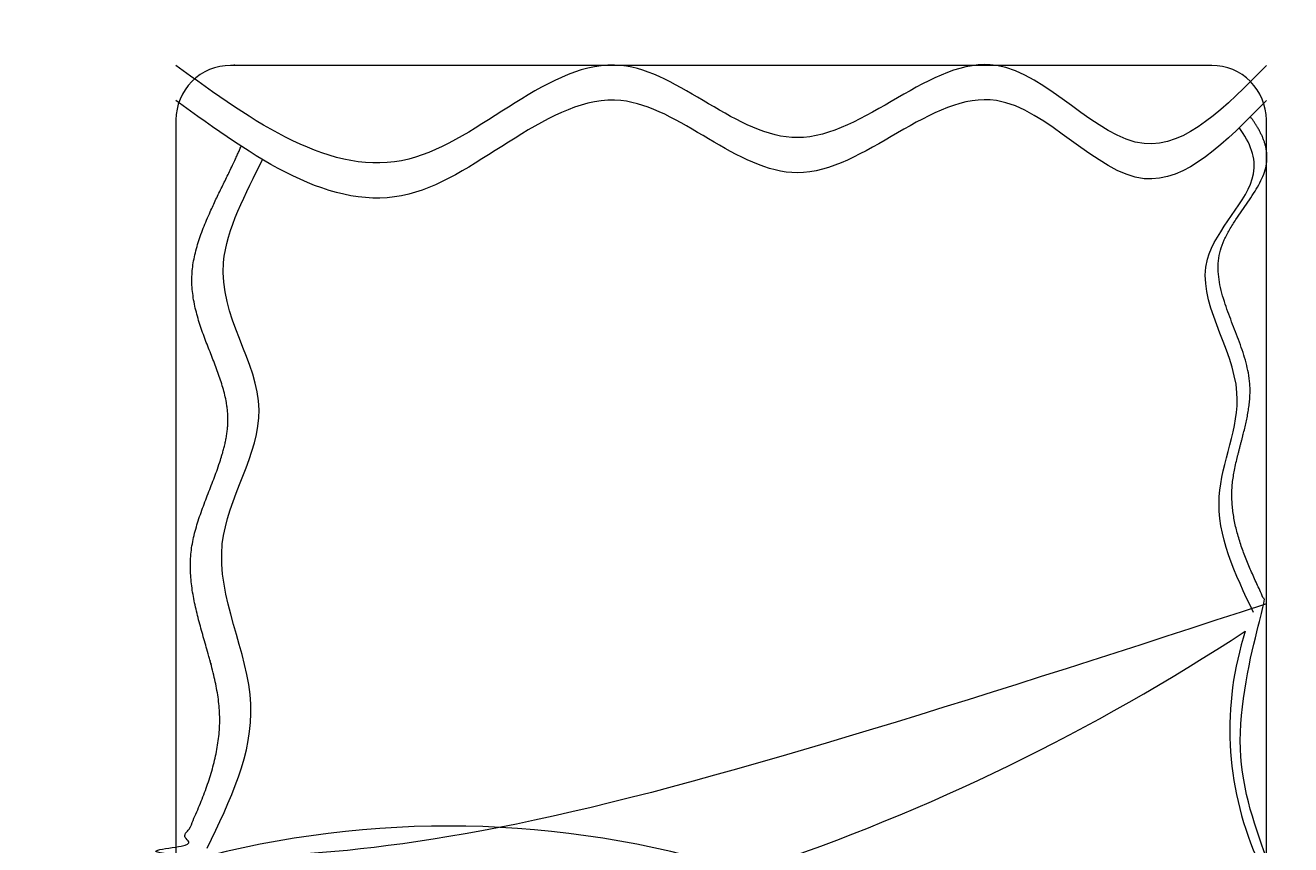
# Model space of a CAD drawing. Units: inches. Extents: x -61 to 1599, y -1316 to 257.
# Tile 39 of 204: x 91 to 171, y -738 to -686. Entities that reach past the tile are written whole.
import ezdxf

# ---------------------------------------------------------------- set-up
doc = ezdxf.new("R2010")
doc.units = ezdxf.units.IN
doc.header["$MEASUREMENT"] = 0
doc.layers.add('A-ANNO-DIMS', color=2, linetype='Continuous', lineweight=18)
doc.layers.add('FURNITURE', color=83, linetype='Continuous', lineweight=18)
doc.styles.get("Standard").update_dxf_attribs({"font": 'arial.ttf'})
doc.dimstyles.get("Standard").update_dxf_attribs({"dimtxt": 0.18, "dimasz": 0.18, "dimexe": 0.18, "dimexo": 0.0625, "dimgap": 0.09, "dimtad": 0, "dimtih": 1, "dimtoh": 1, "dimdec": 0, "dimzin": 0, "dimdsep": 46, "dimlunit": 3, "dimtxsty": 'Standard', "dimcen": 0.09, "dimadec": 0, "dimazin": 0, "dimtfac": 1, "dimtdec": 0, "dimtofl": 0, "dimtmove": 0, "dimatfit": 3, "dimfxl": 1, "dimtolj": 1, "dimtzin": 0, "dimarcsym": 0})

# ---------------------------------------------------------------- blocks, each defined once
blk = doc.blocks.new('BED-DOUBLE')
for points in [[(1.272, 88.537), (1.272, 3.449, 0.414214), (4.722, 0), (66.813, 0, 0.414214), (70.263, 3.449), (70.263, 88.537, 0.414214), (66.813, 91.987), (4.722, 91.987, 0.414214)], [(38.01, 41.126, 0.064396), (68.933, 56.181, 0.181766), (69.614, 41.916, -0.202767)]]:
    blk.add_lwpolyline(points, format="xyb", close=True)
blk.add_lwpolyline([(70.263, 41.387, -0.22309), (35.767, 41.387, 0.142156), (1.272, 41.387)], format="xyb")
for points, knots in [([(70.263, 91.987), (67.707, 89.379), (62.206, 83.764), (52.487, 96.724), (40.92, 82.741), (28.609, 96.737), (15.695, 81.527), (6.205, 88.409), (1.272, 91.987)], [0, 0, 0, 0, 9.176033, 19.753992, 33.150145, 45.209422, 59.881559, 75.764594, 75.764594, 75.764594, 75.764594]), ([(70.263, 89.765), (67.707, 87.157), (62.206, 81.542), (52.487, 94.502), (40.92, 80.519), (28.609, 94.515), (15.695, 79.305), (6.205, 86.187), (1.272, 89.765)], [0, 0, 0, 0, 9.176033, 19.753992, 33.150145, 45.209422, 59.881559, 75.764594, 75.764594, 75.764594, 75.764594]), ([(69.451, 57.362), (68.289, 59.79), (66.113, 64.336), (70.043, 71.905), (64.118, 79.112), (70.314, 84.4), (69.244, 87.088), (68.552, 88.052)], [0, 0, 0, 0, 6.649676, 12.451782, 19.973966, 25.324174, 28.349676, 28.349676, 28.349676, 28.349676]), ([(3.252, 42.437), (4.702, 45.448), (7.724, 51.72), (2.116, 61.25), (8.808, 70.52), (2.434, 77.934), (5.722, 83.908), (6.746, 86.037)], [0, 0, 0, 0, 8.27671, 17.241866, 24.903358, 33.244933, 38.427294, 38.427294, 38.427294, 38.427294])]:
    blk.add_open_spline(points, degree=3, knots=knots)
blk.add_open_spline([(5.011, 91.987), (4.986, 92.006), (4.961, 92.025), (4.936, 92.044)], degree=3)
for points, weights, knots in [([(70.263, 41.825), (68.018, 47.029), (68.018, 52.696), (70.263, 57.9), (69.1, 60.328), (66.924, 64.874), (70.854, 72.444), (64.929, 79.65), (71.186, 84.991), (70.014, 87.727), (69.253, 88.741)], [1, 0.945466318698, 0.945466318698, 1, 1, 1, 1, 1, 1, 1, 1], [0, 0, 0, 0, 0.814571, 0.814571, 0.814571, 7.464247, 13.266353, 20.788537, 26.138745, 29.321895, 29.321895, 29.321895, 29.321895]), ([(70.263, 57.9), (59.862, 50.943), (48.595, 45.5), (36.681, 41.677), (36.463, 41.771), (36.247, 41.868), (36.032, 41.966), (24.597, 45.284), (12.692, 45.258), (1.272, 41.889), (2.723, 44.9), (5.745, 51.172), (0.137, 60.702), (6.828, 69.972), (0.109, 77.787), (4.354, 84.383), (5.398, 86.876)], [1, 0.993520320424, 0.993520320424, 1, 0.99997444972, 0.99997444972, 1, 0.973174868659, 0.973174868659, 1, 1, 1, 1, 1, 1, 1, 1], [0, 0, 0, 0, 0.279074, 0.279074, 0.279074, 0.296584, 0.296584, 0.296584, 0.865868, 0.865868, 0.865868, 9.142578, 18.107734, 25.769226, 34.110801, 40.441511, 40.441511, 40.441511, 40.441511])]:
    blk.add_rational_spline(points, weights, degree=3, knots=knots)
blk = doc.blocks.new('*D687')
at = {"layer": 'A-ANNO-DIMS', "color": 0, "lineweight": -2, "transparency": 16777216}
for p, q in [((289.418, 181.677), (-61.077, 181.677)), ((-60.897, 181.497), (-60.897, -528.952)), ((-60.897, -1239.765), (-60.897, -529.316)), ((319.64, -1239.945), (-61.077, -1239.945))]:
    blk.add_line(p, q, dxfattribs=at)
at = {"layer": 'A-ANNO-DIMS', "color": 0, "transparency": 16777216}
for points in [[(-60.927, 181.497), (-60.867, 181.497), (-60.897, 181.677)], [(-60.927, -1239.765), (-60.867, -1239.765), (-60.897, -1239.945)]]:
    blk.add_solid(points, dxfattribs=at)
at = {"layer": 'DEFPOINTS', "color": 0, "transparency": 16777216}
for p in [(289.481, 181.677), (-60.897, -1239.945), (319.703, -1239.945)]:
    blk.add_point(p, dxfattribs=at)
at = {"layer": 'A-ANNO-DIMS', "color": 0, "transparency": 16777216, "insert": (-60.897, -529.134), "char_height": 0.18, "attachment_point": 5}
blk.add_mtext('\\A1;1421.6', dxfattribs=at)

msp = doc.modelspace()

# ---------------------------------------------------------------- block references
at = {"layer": 'FURNITURE'}
msp.add_blockref('BED-DOUBLE', (98.977, -780.4187), dxfattribs=at)

# ---------------------------------------------------------------- dimensions: what is measured, and where the dimension line sits
at = {"layer": 'A-ANNO-DIMS'}
dim = msp.add_linear_dim(base=(-60.8972, -1239.9446), p1=(289.4807, 181.6771), p2=(319.7028, -1239.9446), angle=90, dimstyle='Standard', override={"dimdec": 1, "dimlfac": 1, "dimrnd": 0, "dimzin": 0, "dimdsep": 46, "dimlunit": 2}, dxfattribs=at)
dim.commit()
dim.dimension.update_dxf_attribs({"geometry": '*D687', "text_midpoint": (-60.8972, -529.1337)})

doc.saveas('drawing.dxf')
